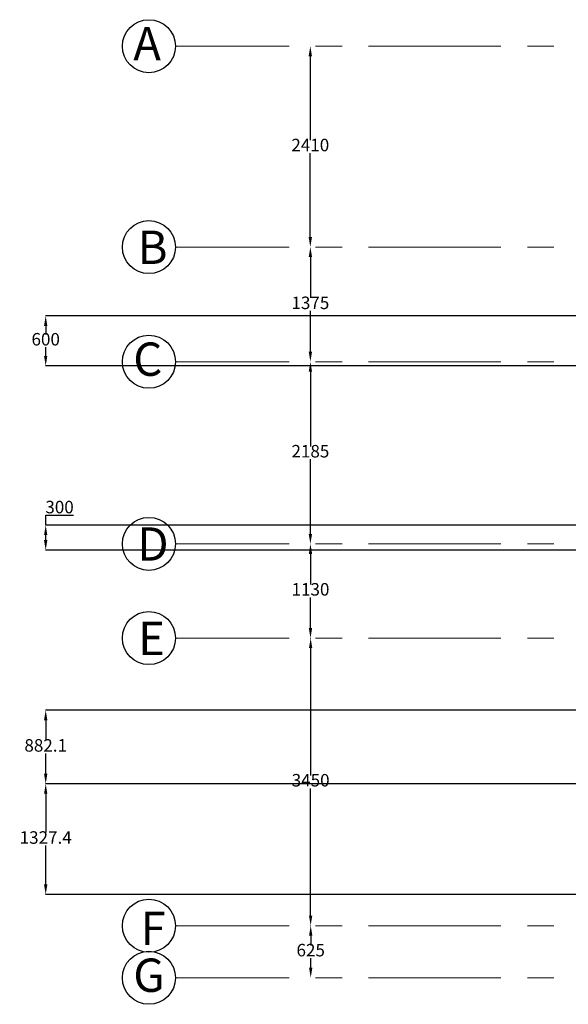
# Model space of a CAD drawing. Units: millimetres. Extents: x -174 to 32373, y 27344 to 53129.
# Tile 3 of 7: x 1623 to 8204, y 37576 to 49387. Entities that reach past the tile are written whole.
import ezdxf

# ---------------------------------------------------------------- set-up
doc = ezdxf.new("R2010")
doc.units = ezdxf.units.MM
doc.header["$LTSCALE"] = 50
doc.linetypes.add('CENTER', pattern=[50.8, 31.75, -6.35, 6.35, -6.35])
for name, color, linetype, lineweight in [('S-ANNO-DIMS', 2, 'Continuous', 18), ('S-GRID', 8, 'CENTER', 18), ('S-GRID-IDEN', 7, 'Continuous', 25)]:
    doc.layers.add(name, color=color, linetype=linetype, lineweight=lineweight)
doc.styles.get("Standard").update_dxf_attribs({"font": 'arial.ttf'})
doc.dimstyles.new('ISO-25', dxfattribs={"dimtxt": 150, "dimasz": 120, "dimexe": 1.25, "dimexo": 0.625, "dimtad": 1, "dimtih": 1, "dimtoh": 1, "dimdec": 0, "dimtxsty": 'Standard', "dimcen": 2.5, "dimadec": 0, "dimazin": 0, "dimtfac": 1, "dimtdec": 0, "dimtmove": 0, "dimatfit": 3, "dimfxl": 1, "dimarcsym": 0})

# ---------------------------------------------------------------- blocks, each defined once
blk = doc.blocks.new('*D10')
at = {"layer": 'Defpoints', "color": 0, "transparency": 16777216}
for p in [(5109, 49069), (5109, 46659), (5109, 46659)]:
    blk.add_point(p, dxfattribs=at)
at = {"layer": 'S-ANNO-DIMS', "color": 0, "lineweight": -2, "transparency": 16777216}
for p, q in [((5110, 49069), (5111, 49069)), ((5109, 48949), (5109, 47941)), ((5109, 46779), (5109, 47787)), ((5110, 46659), (5111, 46659))]:
    blk.add_line(p, q, dxfattribs=at)
at = {"layer": 'S-ANNO-DIMS', "color": 0, "transparency": 16777216}
for points in [[(5089, 48949), (5129, 48949), (5109, 49069)], [(5089, 46779), (5129, 46779), (5109, 46659)]]:
    blk.add_solid(points, dxfattribs=at)
at = {"layer": 'S-ANNO-DIMS', "color": 0, "transparency": 16777216, "insert": (5109, 47864), "char_height": 150, "attachment_point": 5}
blk.add_mtext('2410', dxfattribs=at)
blk = doc.blocks.new('*D11')
at = {"layer": 'Defpoints', "color": 0, "transparency": 16777216}
for p in [(5110, 46659), (5110, 45284), (5110, 45284)]:
    blk.add_point(p, dxfattribs=at)
at = {"layer": 'S-ANNO-DIMS', "color": 0, "lineweight": -2, "transparency": 16777216}
for p, q in [((5111, 46659), (5111, 46659)), ((5110, 46539), (5110, 46049)), ((5110, 45404), (5110, 45894)), ((5111, 45284), (5111, 45284))]:
    blk.add_line(p, q, dxfattribs=at)
at = {"layer": 'S-ANNO-DIMS', "color": 0, "transparency": 16777216}
for points in [[(5090, 46539), (5130, 46539), (5110, 46659)], [(5090, 45404), (5130, 45404), (5110, 45284)]]:
    blk.add_solid(points, dxfattribs=at)
at = {"layer": 'S-ANNO-DIMS', "color": 0, "transparency": 16777216, "insert": (5110, 45971), "char_height": 150, "attachment_point": 5}
blk.add_mtext('1375', dxfattribs=at)
blk = doc.blocks.new('*D12')
at = {"layer": 'Defpoints', "color": 0, "transparency": 16777216}
for p in [(5110, 45284), (5110, 43099), (5110, 43099)]:
    blk.add_point(p, dxfattribs=at)
at = {"layer": 'S-ANNO-DIMS', "color": 0, "lineweight": -2, "transparency": 16777216}
for p, q in [((5111, 45284), (5111, 45284)), ((5110, 45164), (5110, 44268)), ((5110, 43219), (5110, 44114)), ((5111, 43099), (5111, 43099))]:
    blk.add_line(p, q, dxfattribs=at)
at = {"layer": 'S-ANNO-DIMS', "color": 0, "transparency": 16777216}
for points in [[(5090, 45164), (5130, 45164), (5110, 45284)], [(5090, 43219), (5130, 43219), (5110, 43099)]]:
    blk.add_solid(points, dxfattribs=at)
at = {"layer": 'S-ANNO-DIMS', "color": 0, "transparency": 16777216, "insert": (5110, 44191), "char_height": 150, "attachment_point": 5}
blk.add_mtext('2185', dxfattribs=at)
blk = doc.blocks.new('*D13')
at = {"layer": 'Defpoints', "color": 0, "transparency": 16777216}
for p in [(5111, 43099), (5111, 41969), (5111, 41969)]:
    blk.add_point(p, dxfattribs=at)
at = {"layer": 'S-ANNO-DIMS', "color": 0, "lineweight": -2, "transparency": 16777216}
for p, q in [((5112, 43099), (5113, 43099)), ((5111, 42979), (5111, 42611)), ((5111, 42089), (5111, 42456)), ((5112, 41969), (5113, 41969))]:
    blk.add_line(p, q, dxfattribs=at)
at = {"layer": 'S-ANNO-DIMS', "color": 0, "transparency": 16777216}
for points in [[(5091, 42979), (5131, 42979), (5111, 43099)], [(5091, 42089), (5131, 42089), (5111, 41969)]]:
    blk.add_solid(points, dxfattribs=at)
at = {"layer": 'S-ANNO-DIMS', "color": 0, "transparency": 16777216, "insert": (5111, 42534), "char_height": 150, "attachment_point": 5}
blk.add_mtext('1130', dxfattribs=at)
blk = doc.blocks.new('*D14')
at = {"layer": 'Defpoints', "color": 0, "transparency": 16777216}
for p in [(5113, 41969), (5113, 38519), (5113, 38519)]:
    blk.add_point(p, dxfattribs=at)
at = {"layer": 'S-ANNO-DIMS', "color": 0, "lineweight": -2, "transparency": 16777216}
for p, q in [((5113, 41969), (5114, 41969)), ((5113, 41849), (5113, 40321)), ((5113, 38639), (5113, 40166)), ((5113, 38519), (5114, 38519))]:
    blk.add_line(p, q, dxfattribs=at)
at = {"layer": 'S-ANNO-DIMS', "color": 0, "transparency": 16777216}
for points in [[(5093, 41849), (5133, 41849), (5113, 41969)], [(5093, 38639), (5133, 38639), (5113, 38519)]]:
    blk.add_solid(points, dxfattribs=at)
at = {"layer": 'S-ANNO-DIMS', "color": 0, "transparency": 16777216, "insert": (5113, 40244), "char_height": 150, "attachment_point": 5}
blk.add_mtext('3450', dxfattribs=at)
blk = doc.blocks.new('*D15')
at = {"layer": 'Defpoints', "color": 0, "transparency": 16777216}
for p in [(5114, 38519), (5114, 37894), (5114, 37894)]:
    blk.add_point(p, dxfattribs=at)
at = {"layer": 'S-ANNO-DIMS', "color": 0, "lineweight": -2, "transparency": 16777216}
for p, q in [((5114, 38519), (5115, 38519)), ((5114, 38399), (5114, 38283)), ((5114, 38014), (5114, 38129)), ((5114, 37894), (5115, 37894))]:
    blk.add_line(p, q, dxfattribs=at)
at = {"layer": 'S-ANNO-DIMS', "color": 0, "transparency": 16777216}
for points in [[(5094, 38399), (5134, 38399), (5114, 38519)], [(5094, 38014), (5134, 38014), (5114, 37894)]]:
    blk.add_solid(points, dxfattribs=at)
at = {"layer": 'S-ANNO-DIMS', "color": 0, "transparency": 16777216, "insert": (5114, 38206), "char_height": 150, "attachment_point": 5}
blk.add_mtext('625', dxfattribs=at)
blk = doc.blocks.new('*D43')
at = {"layer": 'Defpoints', "color": 0, "transparency": 16777216}
for p in [(1935, 43324), (13627, 43324), (13627, 43024)]:
    blk.add_point(p, dxfattribs=at)
at = {"layer": 'S-ANNO-DIMS', "color": 0, "lineweight": -2, "transparency": 16777216}
for p, q in [((1935, 43324), (1935, 43444)), ((1935, 43444), (2267, 43444)), ((13626, 43324), (1934, 43324)), ((1935, 43144), (1935, 43204)), ((13626, 43024), (1934, 43024))]:
    blk.add_line(p, q, dxfattribs=at)
at = {"layer": 'S-ANNO-DIMS', "color": 0, "transparency": 16777216}
for points in [[(1915, 43204), (1955, 43204), (1935, 43324)], [(1915, 43144), (1955, 43144), (1935, 43024)]]:
    blk.add_solid(points, dxfattribs=at)
at = {"layer": 'S-ANNO-DIMS', "color": 0, "transparency": 16777216, "insert": (2101, 43521), "char_height": 150, "attachment_point": 5}
blk.add_mtext('300', dxfattribs=at)
blk = doc.blocks.new('*D45')
at = {"layer": 'Defpoints', "color": 0, "transparency": 16777216}
for p in [(1935, 45834), (13662, 45834), (13662, 45234)]:
    blk.add_point(p, dxfattribs=at)
at = {"layer": 'S-ANNO-DIMS', "color": 0, "lineweight": -2, "transparency": 16777216}
for p, q in [((13661, 45834), (1934, 45834)), ((1935, 45714), (1935, 45611)), ((1935, 45354), (1935, 45457)), ((13661, 45234), (1934, 45234))]:
    blk.add_line(p, q, dxfattribs=at)
at = {"layer": 'S-ANNO-DIMS', "color": 0, "transparency": 16777216}
for points in [[(1915, 45714), (1955, 45714), (1935, 45834)], [(1915, 45354), (1955, 45354), (1935, 45234)]]:
    blk.add_solid(points, dxfattribs=at)
at = {"layer": 'S-ANNO-DIMS', "color": 0, "transparency": 16777216, "insert": (1935, 45534), "char_height": 150, "attachment_point": 5}
blk.add_mtext('600', dxfattribs=at)
blk = doc.blocks.new('*D56')
at = {"layer": 'Defpoints', "color": 0, "transparency": 16777216}
for p in [(1935, 40221), (8452, 40221), (8452, 38894)]:
    blk.add_point(p, dxfattribs=at)
at = {"layer": 'S-ANNO-DIMS', "color": 0, "lineweight": -2, "transparency": 16777216}
for p, q in [((8451, 40221), (1934, 40221)), ((1935, 40101), (1935, 39635)), ((1935, 39014), (1935, 39480)), ((8451, 38894), (1934, 38894))]:
    blk.add_line(p, q, dxfattribs=at)
at = {"layer": 'S-ANNO-DIMS', "color": 0, "transparency": 16777216}
for points in [[(1915, 40101), (1955, 40101), (1935, 40221)], [(1915, 39014), (1955, 39014), (1935, 38894)]]:
    blk.add_solid(points, dxfattribs=at)
at = {"layer": 'S-ANNO-DIMS', "color": 0, "transparency": 16777216, "insert": (1935, 39557), "char_height": 150, "attachment_point": 5}
blk.add_mtext('1327.4', dxfattribs=at)
blk = doc.blocks.new('*D57')
at = {"layer": 'Defpoints', "color": 0, "transparency": 16777216}
for p in [(1935, 41103), (8452, 41103), (8452, 40221)]:
    blk.add_point(p, dxfattribs=at)
at = {"layer": 'S-ANNO-DIMS', "color": 0, "lineweight": -2, "transparency": 16777216}
for p, q in [((8451, 41103), (1934, 41103)), ((1935, 40983), (1935, 40739)), ((1935, 40341), (1935, 40585)), ((8451, 40221), (1934, 40221))]:
    blk.add_line(p, q, dxfattribs=at)
at = {"layer": 'S-ANNO-DIMS', "color": 0, "transparency": 16777216}
for points in [[(1915, 40983), (1955, 40983), (1935, 41103)], [(1915, 40341), (1955, 40341), (1935, 40221)]]:
    blk.add_solid(points, dxfattribs=at)
at = {"layer": 'S-ANNO-DIMS', "color": 0, "transparency": 16777216, "insert": (1935, 40662), "char_height": 150, "attachment_point": 5}
blk.add_mtext('882.1', dxfattribs=at)

msp = doc.modelspace()

# ---------------------------------------------------------------- linework, layer by layer
at = {"layer": 'S-GRID'}
for p, q in [((20095.15, 49068.76), (3491.75, 49068.76)), ((20095.15, 46658.76), (3491.75, 46658.76)), ((20095.15, 45283.76), (3491.75, 45283.76)), ((20095.15, 43098.76), (3491.75, 43098.76)), ((20095.15, 41968.76), (3491.75, 41968.76)), ((20095.15, 38518.76), (3491.75, 38518.76)), ((20095.15, 37893.76), (3491.75, 37893.76))]:
    msp.add_line(p, q, dxfattribs=at)
at = {"layer": 'S-GRID-IDEN'}
for centre in [(3173.56, 49068.76), (3173.56, 46658.76), (3173.56, 45283.76), (3173.56, 43098.76), (3173.56, 41968.76), (3173.56, 38518.76), (3173.56, 37893.76)]:
    msp.add_circle(centre, 318.18, dxfattribs=at)

# ---------------------------------------------------------------- texts
at = {"layer": 'S-GRID-IDEN', "char_height": 400, "attachment_point": 1}
for s, insert in [('A', (2985.55, 49299.65)), ('B', (3038.28, 46856.72)), ('C', (2985.55, 45514.65)), ('D', (3034.09, 43297.31)), ('E', (3042.85, 42164.32)), ('F', (3073.24, 38686.31)), ('G', (2985.55, 38124.65))]:
    msp.add_mtext_dynamic_manual_height_columns(s, width=343.3972, gutter_width=12.5, heights=[0], dxfattribs=dict(at, insert=insert))

# ---------------------------------------------------------------- dimensions: what is measured, and where the dimension line sits
at = {"layer": 'S-ANNO-DIMS'}
for base, p1, p2, override, picture, middle in [((5109.42, 46658.76), (5109.42, 49068.76), (5109.42, 46658.76), {"dimclrd": 0, "dimclre": 0, "dimclrt": 0}, '*D10', (5109.42, 47863.76)), ((5110.04, 45283.76), (5110.04, 46658.76), (5110.04, 45283.76), {"dimclrd": 0, "dimclre": 0, "dimclrt": 0}, '*D11', (5110.04, 45971.26)), ((1935.38, 45833.76), (13661.66, 45233.76), (13661.66, 45833.76), {"dimdec": 0, "dimlfac": 1, "dimrnd": 0, "dimzin": 0, "dimdsep": 46, "dimlunit": 2}, '*D45', (1935.38, 45533.76)), ((5110.04, 43098.76), (5110.04, 45283.76), (5110.04, 43098.76), {"dimclrd": 0, "dimclre": 0, "dimclrt": 0}, '*D12', (5110.04, 44191.26)), ((1935.38, 43323.76), (13626.66, 43023.76), (13626.66, 43323.76), {"dimdec": 0, "dimlfac": 1, "dimrnd": 0, "dimzin": 0, "dimdsep": 46, "dimlunit": 2}, '*D43', (2101.4, 43521.02)), ((5111.29, 41968.76), (5111.29, 43098.76), (5111.29, 41968.76), {"dimclrd": 0, "dimclre": 0, "dimclrt": 0}, '*D13', (5111.29, 42533.76)), ((5112.54, 38518.76), (5112.54, 41968.76), (5112.54, 38518.76), {"dimclrd": 0, "dimclre": 0, "dimclrt": 0}, '*D14', (5112.54, 40243.76)), ((1935.38, 41103.32), (8451.66, 40221.18), (8451.66, 41103.32), {"dimdec": 1, "dimlfac": 1, "dimrnd": 0, "dimzin": 0, "dimdsep": 46, "dimlunit": 2}, '*D57', (1935.38, 40662.25)), ((1935.38, 40221.18), (8451.66, 38893.76), (8451.66, 40221.18), {"dimdec": 1, "dimlfac": 1, "dimrnd": 0, "dimzin": 0, "dimdsep": 46, "dimlunit": 2}, '*D56', (1935.38, 39557.47)), ((5113.79, 37893.76), (5113.79, 38518.76), (5113.79, 37893.76), {"dimclrd": 0, "dimclre": 0, "dimclrt": 0}, '*D15', (5113.79, 38206.26))]:
    dim = msp.add_linear_dim(base=base, p1=p1, p2=p2, angle=90, dimstyle='ISO-25', override=override, dxfattribs=at)
    dim.commit()
    dim.dimension.update_dxf_attribs({"geometry": picture, "text_midpoint": middle})

doc.saveas('drawing.dxf')
